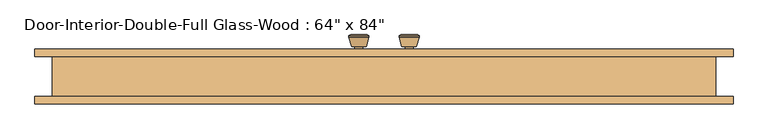
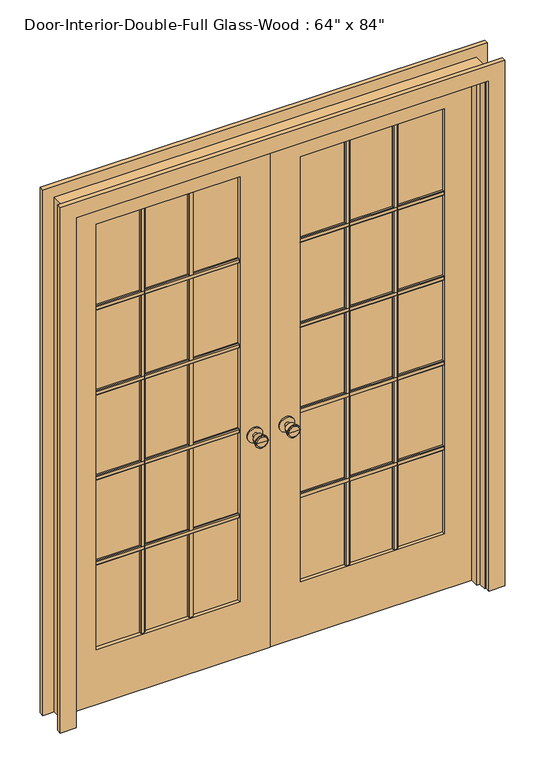
"""IFC4 building model written with IfcOpenShell, lengths in millimetres: door geometry."""

from ifc_helpers import new_model, si_unit, point, frame, frame_2d, origin, place, context, project, spatial, polyline, circle_curve, trimmed, segment, composite_curve, outline, extrude, faceted_brep, source, transform, mapped, element, save
from ifc_brep_helpers import plane_surface, cylinder_surface, revolved_surface, advanced_brep


def door_09c896ac(model_context):
    return source(origin(), model_context, "Body", "SolidModel", [
        advanced_brep(
        [(-63.5, 53.625, 914.4), (-73.5, 53.625, 914.4), (-53.5, 53.625, 914.4), (-83.9758676, 102.625, 914.4), (-63.5, 102.625, 914.4), (-43.0241324, 102.625, 914.4), (-88.5, 100.7971319, 914.4), (-38.5, 100.7971319, 914.4), (-88.5, 97.3334537, 914.4), (-38.5, 97.3334537, 914.4), (-82.136236, 72.625, 914.4), (-44.863764, 72.625, 914.4), (-73.5, 72.625, 914.4), (-53.5, 72.625, 914.4)],
        [
            (0, 1),
            (1, 2, circle_curve(frame((-63.5, 53.625, 914.4), z_axis=(0.0, -1.0, 0.0), x_axis=(1.0, 0.0, 0.0)), 10.0)),
            (2, 0),
            (2, 1, circle_curve(frame((-63.5, 53.625, 914.4), z_axis=(0.0, -1.0, 0.0), x_axis=(1.0, 0.0, 0.0)), 10.0)),
            (3, 4),
            (4, 5),
            (5, 3, circle_curve(frame((-63.5, 102.625, 914.4), z_axis=(0.0, 1.0, 0.0), x_axis=(1.0, 0.0, 0.0)), 20.4758676)),
            (3, 5, circle_curve(frame((-63.5, 102.625, 914.4), z_axis=(0.0, 1.0, 0.0), x_axis=(1.0, 0.0, 0.0)), 20.4758676)),
            (6, 3),
            (5, 7),
            (7, 6, circle_curve(frame((-63.5, 100.7971319, 914.4), z_axis=(0.0, 1.0, 0.0), x_axis=(1.0, 0.0, 0.0)), 25.0)),
            (6, 7, circle_curve(frame((-63.5, 100.7971319, 914.4), z_axis=(0.0, 1.0, 0.0), x_axis=(1.0, 0.0, 0.0)), 25.0)),
            (8, 6),
            (7, 9),
            (9, 8, circle_curve(frame((-63.5, 97.3334537, 914.4), z_axis=(0.0, 1.0, 0.0), x_axis=(1.0, 0.0, 0.0)), 25.0)),
            (8, 9, circle_curve(frame((-63.5, 97.3334537, 914.4), z_axis=(0.0, 1.0, 0.0), x_axis=(1.0, 0.0, 0.0)), 25.0)),
            (10, 8),
            (9, 11),
            (11, 10, circle_curve(frame((-63.5, 72.625, 914.4), z_axis=(0.0, 1.0, 0.0), x_axis=(1.0, 0.0, 0.0)), 18.636236)),
            (10, 11, circle_curve(frame((-63.5, 72.625, 914.4), z_axis=(0.0, 1.0, 0.0), x_axis=(1.0, 0.0, 0.0)), 18.636236)),
            (12, 10),
            (11, 13),
            (13, 12, circle_curve(frame((-63.5, 72.625, 914.4), z_axis=(0.0, 1.0, 0.0), x_axis=(1.0, 0.0, 0.0)), 10.0)),
            (12, 13, circle_curve(frame((-63.5, 72.625, 914.4), z_axis=(0.0, 1.0, 0.0), x_axis=(1.0, 0.0, 0.0)), 10.0)),
            (1, 12),
            (13, 2),
        ],
        [
            plane_surface(frame((-63.5, 53.625, 914.4), z_axis=(0.0, -1.0, 0.0), x_axis=(1.0, 0.0, 0.0))),
            plane_surface(frame((-63.5, 102.625, 914.4), z_axis=(0.0, 1.0, 0.0), x_axis=(1.0, 0.0, 0.0))),
            revolved_surface(polyline([(-43.0241324, 102.625, 914.4), (-38.5, 100.7971319, 914.4)]), (-63.5, 53.625, 914.4), (0.0, -1.0, 0.0)),
            cylinder_surface(frame((-63.5, 53.625, 914.4), z_axis=(0.0, -1.0, 0.0), x_axis=(1.0, 0.0, 0.0)), 25.0),
            revolved_surface(polyline([(-38.5, 97.3334537, 914.4), (-44.863764, 72.625, 914.4)]), (-63.5, 53.625, 914.4), (0.0, -1.0, 0.0)),
            plane_surface(frame((-63.5, 72.625, 914.4), z_axis=(0.0, -1.0, 0.0), x_axis=(1.0, 0.0, 0.0))),
            cylinder_surface(frame((-63.5, 53.625, 914.4), z_axis=(0.0, -1.0, 0.0), x_axis=(1.0, 0.0, 0.0)), 10.0),
        ],
        [
            (0, [[1, 2, 3]]),
            (0, [[-3, 4, -1]]),
            (1, [[5, 6, 7]]),
            (1, [[-6, -5, 8]]),
            (2, [[9, -7, 10, 11]]),
            (2, [[-10, -8, -9, 12]]),
            (3, [[13, -11, 14, 15]]),
            (3, [[-14, -12, -13, 16]]),
            (4, [[17, -15, 18, 19]]),
            (4, [[-18, -16, -17, 20]]),
            (5, [[21, -19, 22, 23]]),
            (5, [[-22, -20, -21, 24]]),
            (6, [[25, -23, 26, -2]]),
            (6, [[-26, -24, -25, -4]]),
        ],
    ),
        extrude(outline(composite_curve([segment(trimmed(circle_curve(frame_2d((914.4, -63.5)), 30.0), [point((914.4, -33.5))], [point((914.4, -93.5))], False, "CARTESIAN"), True, "CONTINUOUS"), segment(trimmed(circle_curve(frame_2d((914.4, -63.5)), 30.0), [point((914.4, -93.5))], [point((914.4, -33.5))], False, "CARTESIAN"), True, "CONTINUOUS")], self_intersect=False)), frame((0.0, 47.625, 0.0), z_axis=(0.0, 1.0, 0.0), x_axis=(0.0, 0.0, 1.0)), (0.0, 0.0, 1.0), 6.0),
        advanced_brep(
        [(-63.5, 6.7, 914.4), (-53.5, 6.7, 914.4), (-73.5, 6.7, 914.4), (-83.9758676, -42.3, 914.4), (-43.0241324, -42.3, 914.4), (-63.5, -42.3, 914.4), (-88.5, -40.4721319, 914.4), (-38.5, -40.4721319, 914.4), (-88.5, -37.0084537, 914.4), (-38.5, -37.0084537, 914.4), (-82.136236, -12.3, 914.4), (-44.863764, -12.3, 914.4), (-73.5, -12.3, 914.4), (-53.5, -12.3, 914.4)],
        [
            (0, 1),
            (1, 2, circle_curve(frame((-63.5, 6.7, 914.4), z_axis=(0.0, 1.0, 0.0), x_axis=(1.0, 0.0, 0.0)), 10.0)),
            (2, 0),
            (2, 1, circle_curve(frame((-63.5, 6.7, 914.4), z_axis=(0.0, 1.0, 0.0), x_axis=(1.0, 0.0, 0.0)), 10.0)),
            (3, 4, circle_curve(frame((-63.5, -42.3, 914.4), z_axis=(0.0, -1.0, 0.0), x_axis=(1.0, 0.0, 0.0)), 20.4758676)),
            (4, 5),
            (5, 3),
            (4, 3, circle_curve(frame((-63.5, -42.3, 914.4), z_axis=(0.0, -1.0, 0.0), x_axis=(1.0, 0.0, 0.0)), 20.4758676)),
            (6, 7, circle_curve(frame((-63.5, -40.4721319, 914.4), z_axis=(0.0, -1.0, 0.0), x_axis=(1.0, 0.0, 0.0)), 25.0)),
            (7, 4),
            (3, 6),
            (7, 6, circle_curve(frame((-63.5, -40.4721319, 914.4), z_axis=(0.0, -1.0, 0.0), x_axis=(1.0, 0.0, 0.0)), 25.0)),
            (8, 9, circle_curve(frame((-63.5, -37.0084537, 914.4), z_axis=(0.0, -1.0, 0.0), x_axis=(1.0, 0.0, 0.0)), 25.0)),
            (9, 7),
            (6, 8),
            (9, 8, circle_curve(frame((-63.5, -37.0084537, 914.4), z_axis=(0.0, -1.0, 0.0), x_axis=(1.0, 0.0, 0.0)), 25.0)),
            (10, 11, circle_curve(frame((-63.5, -12.3, 914.4), z_axis=(0.0, -1.0, 0.0), x_axis=(1.0, 0.0, 0.0)), 18.636236)),
            (11, 9),
            (8, 10),
            (11, 10, circle_curve(frame((-63.5, -12.3, 914.4), z_axis=(0.0, -1.0, 0.0), x_axis=(1.0, 0.0, 0.0)), 18.636236)),
            (12, 13, circle_curve(frame((-63.5, -12.3, 914.4), z_axis=(0.0, -1.0, 0.0), x_axis=(1.0, 0.0, 0.0)), 10.0)),
            (13, 11),
            (10, 12),
            (13, 12, circle_curve(frame((-63.5, -12.3, 914.4), z_axis=(0.0, -1.0, 0.0), x_axis=(1.0, 0.0, 0.0)), 10.0)),
            (1, 13),
            (12, 2),
        ],
        [
            plane_surface(frame((-63.5, 6.7, 914.4), z_axis=(0.0, 1.0, 0.0), x_axis=(1.0, 0.0, 0.0))),
            plane_surface(frame((-63.5, -42.3, 914.4), z_axis=(0.0, -1.0, 0.0), x_axis=(1.0, 0.0, 0.0))),
            revolved_surface(polyline([(-43.0241324, -42.3, 914.4), (-38.5, -40.4721319, 914.4)]), (-63.5, 6.7, 914.4), (0.0, 1.0, 0.0)),
            cylinder_surface(frame((-63.5, 6.7, 914.4), z_axis=(0.0, 1.0, 0.0), x_axis=(1.0, 0.0, 0.0)), 25.0),
            revolved_surface(polyline([(-38.5, -37.0084537, 914.4), (-44.863764, -12.3, 914.4)]), (-63.5, 6.7, 914.4), (0.0, 1.0, 0.0)),
            plane_surface(frame((-63.5, -12.3, 914.4), z_axis=(0.0, 1.0, 0.0), x_axis=(1.0, 0.0, 0.0))),
            cylinder_surface(frame((-63.5, 6.7, 914.4), z_axis=(0.0, 1.0, 0.0), x_axis=(1.0, 0.0, 0.0)), 10.0),
        ],
        [
            (0, [[1, 2, 3]]),
            (0, [[-3, 4, -1]]),
            (1, [[5, 6, 7]]),
            (1, [[8, -7, -6]]),
            (2, [[9, 10, -5, 11]]),
            (2, [[12, -11, -8, -10]]),
            (3, [[13, 14, -9, 15]]),
            (3, [[16, -15, -12, -14]]),
            (4, [[17, 18, -13, 19]]),
            (4, [[20, -19, -16, -18]]),
            (5, [[21, 22, -17, 23]]),
            (5, [[24, -23, -20, -22]]),
            (6, [[-2, 25, -21, 26]]),
            (6, [[-4, -26, -24, -25]]),
        ],
    ),
        extrude(outline(composite_curve([segment(trimmed(circle_curve(frame_2d((914.4, -63.5)), 30.0), [point((914.4, -33.5))], [point((914.4, -93.5))], False, "CARTESIAN"), True, "CONTINUOUS"), segment(trimmed(circle_curve(frame_2d((914.4, -63.5)), 30.0), [point((914.4, -93.5))], [point((914.4, -33.5))], False, "CARTESIAN"), True, "CONTINUOUS")], self_intersect=False)), frame((0.0, 6.7, 0.0), z_axis=(0.0, 1.0, 0.0), x_axis=(0.0, 0.0, 1.0)), (0.0, 0.0, 1.0), 6.0),
        extrude(outline(polyline([(26.67, 1667.51), (26.67, 1648.46), (20.32, 1648.46), (17.145, 1651.635), (17.145, 1664.335), (20.32, 1667.51), (26.67, 1667.51)])), frame((120.65, 0.0, 0.0), z_axis=(1.0, 0.0, 0.0), x_axis=(0.0, 1.0, 0.0)), (0.0, 0.0, 1.0), 571.5),
        extrude(outline(polyline([(26.67, 1310.9575), (26.67, 1291.9075), (20.32, 1291.9075), (17.145, 1295.0825), (17.145, 1307.7825), (20.32, 1310.9575), (26.67, 1310.9575)])), frame((120.65, 0.0, 0.0), z_axis=(1.0, 0.0, 0.0), x_axis=(0.0, 1.0, 0.0)), (0.0, 0.0, 1.0), 571.5),
        extrude(outline(polyline([(26.67, 954.405), (26.67, 935.355), (20.32, 935.355), (17.145, 938.53), (17.145, 951.23), (20.32, 954.405), (26.67, 954.405)])), frame((120.65, 0.0, 0.0), z_axis=(1.0, 0.0, 0.0), x_axis=(0.0, 1.0, 0.0)), (0.0, 0.0, 1.0), 571.5),
        extrude(outline(polyline([(26.67, 597.8525), (26.67, 578.8025), (20.32, 578.8025), (17.145, 581.9775), (17.145, 594.6775), (20.32, 597.8525), (26.67, 597.8525)])), frame((120.65, 0.0, 0.0), z_axis=(1.0, 0.0, 0.0), x_axis=(0.0, 1.0, 0.0)), (0.0, 0.0, 1.0), 571.5),
        extrude(outline(polyline([(492.125, 26.67), (511.175, 26.67), (511.175, 20.32), (508.0, 17.145), (495.3, 17.145), (492.125, 20.32), (492.125, 26.67)])), frame((0.0, 0.0, 231.775), z_axis=(0.0, 0.0, 1.0), x_axis=(1.0, 0.0, 0.0)), (0.0, 0.0, 1.0), 1782.7625),
        extrude(outline(polyline([(301.625, 26.67), (320.675, 26.67), (320.675, 20.32), (317.5, 17.145), (304.8, 17.145), (301.625, 20.32), (301.625, 26.67)])), frame((0.0, 0.0, 231.775), z_axis=(0.0, 0.0, 1.0), x_axis=(1.0, 0.0, 0.0)), (0.0, 0.0, 1.0), 1782.7625),
        extrude(outline(polyline([(33.655, 1667.51), (40.005, 1667.51), (43.18, 1664.335), (43.18, 1651.635), (40.005, 1648.46), (33.655, 1648.46), (33.655, 1667.51)])), frame((-692.15, 0.0, 0.0), z_axis=(1.0, 0.0, 0.0), x_axis=(0.0, 1.0, 0.0)), (0.0, 0.0, 1.0), 571.5),
        extrude(outline(polyline([(33.655, 1310.9575), (40.005, 1310.9575), (43.18, 1307.7825), (43.18, 1295.0825), (40.005, 1291.9075), (33.655, 1291.9075), (33.655, 1310.9575)])), frame((-692.15, 0.0, 0.0), z_axis=(1.0, 0.0, 0.0), x_axis=(0.0, 1.0, 0.0)), (0.0, 0.0, 1.0), 571.5),
        extrude(outline(polyline([(33.655, 954.405), (40.005, 954.405), (43.18, 951.23), (43.18, 938.53), (40.005, 935.355), (33.655, 935.355), (33.655, 954.405)])), frame((-692.15, 0.0, 0.0), z_axis=(1.0, 0.0, 0.0), x_axis=(0.0, 1.0, 0.0)), (0.0, 0.0, 1.0), 571.5),
        extrude(outline(polyline([(33.655, 597.8525), (40.005, 597.8525), (43.18, 594.6775), (43.18, 581.9775), (40.005, 578.8025), (33.655, 578.8025), (33.655, 597.8525)])), frame((-692.15, 0.0, 0.0), z_axis=(1.0, 0.0, 0.0), x_axis=(0.0, 1.0, 0.0)), (0.0, 0.0, 1.0), 571.5),
        extrude(outline(polyline([(-320.675, 33.655), (-320.675, 40.005), (-317.5, 43.18), (-304.8, 43.18), (-301.625, 40.005), (-301.625, 33.655), (-320.675, 33.655)])), frame((0.0, 0.0, 231.775), z_axis=(0.0, 0.0, 1.0), x_axis=(1.0, 0.0, 0.0)), (0.0, 0.0, 1.0), 1782.7625),
        extrude(outline(polyline([(-511.175, 33.655), (-511.175, 40.005), (-508.0, 43.18), (-495.3, 43.18), (-492.125, 40.005), (-492.125, 33.655), (-511.175, 33.655)])), frame((0.0, 0.0, 231.775), z_axis=(0.0, 0.0, 1.0), x_axis=(1.0, 0.0, 0.0)), (0.0, 0.0, 1.0), 1782.7625),
        extrude(outline(polyline([(33.655, 1667.51), (40.005, 1667.51), (43.18, 1664.335), (43.18, 1651.635), (40.005, 1648.46), (33.655, 1648.46), (33.655, 1667.51)])), frame((120.65, 0.0, 0.0), z_axis=(1.0, 0.0, 0.0), x_axis=(0.0, 1.0, 0.0)), (0.0, 0.0, 1.0), 571.5),
        extrude(outline(polyline([(33.655, 1310.9575), (40.005, 1310.9575), (43.18, 1307.7825), (43.18, 1295.0825), (40.005, 1291.9075), (33.655, 1291.9075), (33.655, 1310.9575)])), frame((120.65, 0.0, 0.0), z_axis=(1.0, 0.0, 0.0), x_axis=(0.0, 1.0, 0.0)), (0.0, 0.0, 1.0), 571.5),
        extrude(outline(polyline([(33.655, 954.405), (40.005, 954.405), (43.18, 951.23), (43.18, 938.53), (40.005, 935.355), (33.655, 935.355), (33.655, 954.405)])), frame((120.65, 0.0, 0.0), z_axis=(1.0, 0.0, 0.0), x_axis=(0.0, 1.0, 0.0)), (0.0, 0.0, 1.0), 571.5),
        extrude(outline(polyline([(33.655, 597.8525), (40.005, 597.8525), (43.18, 594.6775), (43.18, 581.9775), (40.005, 578.8025), (33.655, 578.8025), (33.655, 597.8525)])), frame((120.65, 0.0, 0.0), z_axis=(1.0, 0.0, 0.0), x_axis=(0.0, 1.0, 0.0)), (0.0, 0.0, 1.0), 571.5),
        extrude(outline(polyline([(492.125, 33.655), (492.125, 40.005), (495.3, 43.18), (508.0, 43.18), (511.175, 40.005), (511.175, 33.655), (492.125, 33.655)])), frame((0.0, 0.0, 231.775), z_axis=(0.0, 0.0, 1.0), x_axis=(1.0, 0.0, 0.0)), (0.0, 0.0, 1.0), 1782.7625),
        extrude(outline(polyline([(301.625, 33.655), (301.625, 40.005), (304.8, 43.18), (317.5, 43.18), (320.675, 40.005), (320.675, 33.655), (301.625, 33.655)])), frame((0.0, 0.0, 231.775), z_axis=(0.0, 0.0, 1.0), x_axis=(1.0, 0.0, 0.0)), (0.0, 0.0, 1.0), 1782.7625),
        extrude(outline(polyline([(26.67, 1667.51), (26.67, 1648.46), (20.32, 1648.46), (17.145, 1651.635), (17.145, 1664.335), (20.32, 1667.51), (26.67, 1667.51)])), frame((-692.15, 0.0, 0.0), z_axis=(1.0, 0.0, 0.0), x_axis=(0.0, 1.0, 0.0)), (0.0, 0.0, 1.0), 571.5),
        extrude(outline(polyline([(26.67, 1310.9575), (26.67, 1291.9075), (20.32, 1291.9075), (17.145, 1295.0825), (17.145, 1307.7825), (20.32, 1310.9575), (26.67, 1310.9575)])), frame((-692.15, 0.0, 0.0), z_axis=(1.0, 0.0, 0.0), x_axis=(0.0, 1.0, 0.0)), (0.0, 0.0, 1.0), 571.5),
        extrude(outline(polyline([(26.67, 954.405), (26.67, 935.355), (20.32, 935.355), (17.145, 938.53), (17.145, 951.23), (20.32, 954.405), (26.67, 954.405)])), frame((-692.15, 0.0, 0.0), z_axis=(1.0, 0.0, 0.0), x_axis=(0.0, 1.0, 0.0)), (0.0, 0.0, 1.0), 571.5),
        extrude(outline(polyline([(26.67, 597.8525), (26.67, 578.8025), (20.32, 578.8025), (17.145, 581.9775), (17.145, 594.6775), (20.32, 597.8525), (26.67, 597.8525)])), frame((-692.15, 0.0, 0.0), z_axis=(1.0, 0.0, 0.0), x_axis=(0.0, 1.0, 0.0)), (0.0, 0.0, 1.0), 571.5),
        extrude(outline(polyline([(-320.675, 26.67), (-301.625, 26.67), (-301.625, 20.32), (-304.8, 17.145), (-317.5, 17.145), (-320.675, 20.32), (-320.675, 26.67)])), frame((0.0, 0.0, 231.775), z_axis=(0.0, 0.0, 1.0), x_axis=(1.0, 0.0, 0.0)), (0.0, 0.0, 1.0), 1782.7625),
        extrude(outline(polyline([(-511.175, 26.67), (-492.125, 26.67), (-492.125, 20.32), (-495.3, 17.145), (-508.0, 17.145), (-511.175, 20.32), (-511.175, 26.67)])), frame((0.0, 0.0, 231.775), z_axis=(0.0, 0.0, 1.0), x_axis=(1.0, 0.0, 0.0)), (0.0, 0.0, 1.0), 1782.7625),
        advanced_brep(
        [(63.5, 6.7, 914.4), (73.5, 6.7, 914.4), (53.5, 6.7, 914.4), (83.9758676, -42.3, 914.4), (63.5, -42.3, 914.4), (43.0241324, -42.3, 914.4), (88.5, -40.4721319, 914.4), (38.5, -40.4721319, 914.4), (88.5, -37.0084537, 914.4), (38.5, -37.0084537, 914.4), (82.136236, -12.3, 914.4), (44.863764, -12.3, 914.4), (73.5, -12.3, 914.4), (53.5, -12.3, 914.4)],
        [
            (0, 1),
            (1, 2, circle_curve(frame((63.5, 6.7, 914.4), z_axis=(0.0, 1.0, 0.0), x_axis=(-1.0, 0.0, 0.0)), 10.0)),
            (2, 0),
            (2, 1, circle_curve(frame((63.5, 6.7, 914.4), z_axis=(0.0, 1.0, 0.0), x_axis=(-1.0, 0.0, 0.0)), 10.0)),
            (3, 4),
            (4, 5),
            (5, 3, circle_curve(frame((63.5, -42.3, 914.4), z_axis=(0.0, -1.0, 0.0), x_axis=(-1.0, 0.0, 0.0)), 20.4758676)),
            (3, 5, circle_curve(frame((63.5, -42.3, 914.4), z_axis=(0.0, -1.0, 0.0), x_axis=(-1.0, 0.0, 0.0)), 20.4758676)),
            (6, 3),
            (5, 7),
            (7, 6, circle_curve(frame((63.5, -40.4721319, 914.4), z_axis=(0.0, -1.0, 0.0), x_axis=(-1.0, 0.0, 0.0)), 25.0)),
            (6, 7, circle_curve(frame((63.5, -40.4721319, 914.4), z_axis=(0.0, -1.0, 0.0), x_axis=(-1.0, 0.0, 0.0)), 25.0)),
            (8, 6),
            (7, 9),
            (9, 8, circle_curve(frame((63.5, -37.0084537, 914.4), z_axis=(0.0, -1.0, 0.0), x_axis=(-1.0, 0.0, 0.0)), 25.0)),
            (8, 9, circle_curve(frame((63.5, -37.0084537, 914.4), z_axis=(0.0, -1.0, 0.0), x_axis=(-1.0, 0.0, 0.0)), 25.0)),
            (10, 8),
            (9, 11),
            (11, 10, circle_curve(frame((63.5, -12.3, 914.4), z_axis=(0.0, -1.0, 0.0), x_axis=(-1.0, 0.0, 0.0)), 18.636236)),
            (10, 11, circle_curve(frame((63.5, -12.3, 914.4), z_axis=(0.0, -1.0, 0.0), x_axis=(-1.0, 0.0, 0.0)), 18.636236)),
            (12, 10),
            (11, 13),
            (13, 12, circle_curve(frame((63.5, -12.3, 914.4), z_axis=(0.0, -1.0, 0.0), x_axis=(-1.0, 0.0, 0.0)), 10.0)),
            (12, 13, circle_curve(frame((63.5, -12.3, 914.4), z_axis=(0.0, -1.0, 0.0), x_axis=(-1.0, 0.0, 0.0)), 10.0)),
            (1, 12),
            (13, 2),
        ],
        [
            plane_surface(frame((63.5, 6.7, 914.4), z_axis=(0.0, 1.0, 0.0), x_axis=(-1.0, 0.0, 0.0))),
            plane_surface(frame((63.5, -42.3, 914.4), z_axis=(0.0, -1.0, 0.0), x_axis=(-1.0, 0.0, 0.0))),
            revolved_surface(polyline([(43.0241324, -42.3, 914.4), (38.5, -40.4721319, 914.4)]), (63.5, 6.7, 914.4), (0.0, 1.0, 0.0)),
            cylinder_surface(frame((63.5, 6.7, 914.4), z_axis=(0.0, 1.0, 0.0), x_axis=(-1.0, 0.0, 0.0)), 25.0),
            revolved_surface(polyline([(38.5, -37.0084537, 914.4), (44.863764, -12.3, 914.4)]), (63.5, 6.7, 914.4), (0.0, 1.0, 0.0)),
            plane_surface(frame((63.5, -12.3, 914.4), z_axis=(0.0, 1.0, 0.0), x_axis=(-1.0, 0.0, 0.0))),
            cylinder_surface(frame((63.5, 6.7, 914.4), z_axis=(0.0, 1.0, 0.0), x_axis=(-1.0, 0.0, 0.0)), 10.0),
        ],
        [
            (0, [[1, 2, 3]]),
            (0, [[-3, 4, -1]]),
            (1, [[5, 6, 7]]),
            (1, [[-6, -5, 8]]),
            (2, [[9, -7, 10, 11]]),
            (2, [[-10, -8, -9, 12]]),
            (3, [[13, -11, 14, 15]]),
            (3, [[-14, -12, -13, 16]]),
            (4, [[17, -15, 18, 19]]),
            (4, [[-18, -16, -17, 20]]),
            (5, [[21, -19, 22, 23]]),
            (5, [[-22, -20, -21, 24]]),
            (6, [[25, -23, 26, -2]]),
            (6, [[-26, -24, -25, -4]]),
        ],
    ),
        extrude(outline(composite_curve([segment(trimmed(circle_curve(frame_2d((914.4, 63.5)), 30.0), [point((914.4, 33.5))], [point((914.4, 93.5))], False, "CARTESIAN"), True, "CONTINUOUS"), segment(trimmed(circle_curve(frame_2d((914.4, 63.5)), 30.0), [point((914.4, 93.5))], [point((914.4, 33.5))], False, "CARTESIAN"), True, "CONTINUOUS")], self_intersect=False)), frame((0.0, 6.7, 0.0), z_axis=(0.0, 1.0, 0.0), x_axis=(0.0, 0.0, 1.0)), (0.0, 0.0, 1.0), 6.0),
        advanced_brep(
        [(63.5, 53.625, 914.4), (53.5, 53.625, 914.4), (73.5, 53.625, 914.4), (83.9758676, 102.625, 914.4), (43.0241324, 102.625, 914.4), (63.5, 102.625, 914.4), (88.5, 100.7971319, 914.4), (38.5, 100.7971319, 914.4), (88.5, 97.3334537, 914.4), (38.5, 97.3334537, 914.4), (82.136236, 72.625, 914.4), (44.863764, 72.625, 914.4), (73.5, 72.625, 914.4), (53.5, 72.625, 914.4)],
        [
            (0, 1),
            (1, 2, circle_curve(frame((63.5, 53.625, 914.4), z_axis=(0.0, -1.0, 0.0), x_axis=(-1.0, 0.0, 0.0)), 10.0)),
            (2, 0),
            (2, 1, circle_curve(frame((63.5, 53.625, 914.4), z_axis=(0.0, -1.0, 0.0), x_axis=(-1.0, 0.0, 0.0)), 10.0)),
            (3, 4, circle_curve(frame((63.5, 102.625, 914.4), z_axis=(0.0, 1.0, 0.0), x_axis=(-1.0, 0.0, 0.0)), 20.4758676)),
            (4, 5),
            (5, 3),
            (4, 3, circle_curve(frame((63.5, 102.625, 914.4), z_axis=(0.0, 1.0, 0.0), x_axis=(-1.0, 0.0, 0.0)), 20.4758676)),
            (6, 7, circle_curve(frame((63.5, 100.7971319, 914.4), z_axis=(0.0, 1.0, 0.0), x_axis=(-1.0, 0.0, 0.0)), 25.0)),
            (7, 4),
            (3, 6),
            (7, 6, circle_curve(frame((63.5, 100.7971319, 914.4), z_axis=(0.0, 1.0, 0.0), x_axis=(-1.0, 0.0, 0.0)), 25.0)),
            (8, 9, circle_curve(frame((63.5, 97.3334537, 914.4), z_axis=(0.0, 1.0, 0.0), x_axis=(-1.0, 0.0, 0.0)), 25.0)),
            (9, 7),
            (6, 8),
            (9, 8, circle_curve(frame((63.5, 97.3334537, 914.4), z_axis=(0.0, 1.0, 0.0), x_axis=(-1.0, 0.0, 0.0)), 25.0)),
            (10, 11, circle_curve(frame((63.5, 72.625, 914.4), z_axis=(0.0, 1.0, 0.0), x_axis=(-1.0, 0.0, 0.0)), 18.636236)),
            (11, 9),
            (8, 10),
            (11, 10, circle_curve(frame((63.5, 72.625, 914.4), z_axis=(0.0, 1.0, 0.0), x_axis=(-1.0, 0.0, 0.0)), 18.636236)),
            (12, 13, circle_curve(frame((63.5, 72.625, 914.4), z_axis=(0.0, 1.0, 0.0), x_axis=(-1.0, 0.0, 0.0)), 10.0)),
            (13, 11),
            (10, 12),
            (13, 12, circle_curve(frame((63.5, 72.625, 914.4), z_axis=(0.0, 1.0, 0.0), x_axis=(-1.0, 0.0, 0.0)), 10.0)),
            (1, 13),
            (12, 2),
        ],
        [
            plane_surface(frame((63.5, 53.625, 914.4), z_axis=(0.0, -1.0, 0.0), x_axis=(-1.0, 0.0, 0.0))),
            plane_surface(frame((63.5, 102.625, 914.4), z_axis=(0.0, 1.0, 0.0), x_axis=(-1.0, 0.0, 0.0))),
            revolved_surface(polyline([(43.0241324, 102.625, 914.4), (38.5, 100.7971319, 914.4)]), (63.5, 53.625, 914.4), (0.0, -1.0, 0.0)),
            cylinder_surface(frame((63.5, 53.625, 914.4), z_axis=(0.0, -1.0, 0.0), x_axis=(-1.0, 0.0, 0.0)), 25.0),
            revolved_surface(polyline([(38.5, 97.3334537, 914.4), (44.863764, 72.625, 914.4)]), (63.5, 53.625, 914.4), (0.0, -1.0, 0.0)),
            plane_surface(frame((63.5, 72.625, 914.4), z_axis=(0.0, -1.0, 0.0), x_axis=(-1.0, 0.0, 0.0))),
            cylinder_surface(frame((63.5, 53.625, 914.4), z_axis=(0.0, -1.0, 0.0), x_axis=(-1.0, 0.0, 0.0)), 10.0),
        ],
        [
            (0, [[1, 2, 3]]),
            (0, [[-3, 4, -1]]),
            (1, [[5, 6, 7]]),
            (1, [[8, -7, -6]]),
            (2, [[9, 10, -5, 11]]),
            (2, [[12, -11, -8, -10]]),
            (3, [[13, 14, -9, 15]]),
            (3, [[16, -15, -12, -14]]),
            (4, [[17, 18, -13, 19]]),
            (4, [[20, -19, -16, -18]]),
            (5, [[21, 22, -17, 23]]),
            (5, [[24, -23, -20, -22]]),
            (6, [[-2, 25, -21, 26]]),
            (6, [[-4, -26, -24, -25]]),
        ],
    ),
        extrude(outline(composite_curve([segment(trimmed(circle_curve(frame_2d((914.4, 63.5)), 30.0), [point((914.4, 33.5))], [point((914.4, 93.5))], False, "CARTESIAN"), True, "CONTINUOUS"), segment(trimmed(circle_curve(frame_2d((914.4, 63.5)), 30.0), [point((914.4, 93.5))], [point((914.4, 33.5))], False, "CARTESIAN"), True, "CONTINUOUS")], self_intersect=False)), frame((0.0, 47.625, 0.0), z_axis=(0.0, 1.0, 0.0), x_axis=(0.0, 0.0, 1.0)), (0.0, 0.0, 1.0), 6.0),
        extrude(outline(polyline([(0.0, 819.15), (0.0, 882.65), (2203.45, 882.65), (2203.45, -882.65), (0.0, -882.65), (0.0, -819.15), (2139.95, -819.15), (2139.95, 819.15), (0.0, 819.15)])), frame((0.0, -73.025, 0.0), z_axis=(0.0, 1.0, 0.0), x_axis=(0.0, 0.0, 1.0)), (0.0, 0.0, 1.0), 19.05),
        extrude(outline(polyline([(0.0, 819.15), (0.0, 882.65), (2203.45, 882.65), (2203.45, -882.65), (0.0, -882.65), (0.0, -819.15), (2139.95, -819.15), (2139.95, 819.15), (0.0, 819.15)])), frame((0.0, 47.625, 0.0), z_axis=(0.0, 1.0, 0.0), x_axis=(0.0, 0.0, 1.0)), (0.0, 0.0, 1.0), 19.05),
        faceted_brep([(838.2, 47.625, 0.0), (838.2, -53.975, 0.0), (812.8, -53.975, 0.0), (812.8, -22.225, 0.0), (800.1, -22.225, 0.0), (800.1, 12.7, 0.0), (812.8, 12.7, 0.0), (812.8, 47.625, 0.0), (838.2, 47.625, 2159.0), (838.2, -53.975, 2159.0), (-838.2, -53.975, 2159.0), (-838.2, -53.975, 0.0), (-812.8, -53.975, 0.0), (-812.8, -53.975, 2133.6), (812.8, -53.975, 2133.6), (812.8, -22.225, 2133.6), (-812.8, -22.225, 2133.6), (-812.8, -22.225, 0.0), (-800.1, -22.225, 0.0), (-800.1, -22.225, 2120.9), (800.1, -22.225, 2120.9), (800.1, 12.7, 2120.9), (1.5875, 12.7, 2120.9), (-1.6019111, 12.7, 2120.9), (-800.1, 12.7, 2120.9), (-800.1, 12.7, 0.0), (-812.8, 12.7, 0.0), (-812.8, 12.7, 2133.6), (-1.6019111, 12.7, 2133.6), (1.5875, 12.7, 2133.6), (812.8, 12.7, 2133.6), (812.8, 47.625, 2133.6), (1.5875, 47.625, 2133.6), (-1.6019111, 47.625, 2133.6), (-812.8, 47.625, 2133.6), (-812.8, 47.625, 0.0), (-838.2, 47.625, 0.0), (-838.2, 47.625, 2159.0)], [[[0, 1, 2, 3, 4, 5, 6, 7]], [[1, 0, 8, 9]], [[2, 1, 9, 10, 11, 12, 13, 14]], [[3, 2, 14, 15]], [[4, 3, 15, 16, 17, 18, 19, 20]], [[5, 4, 20, 21]], [[6, 5, 21, 22, 23, 24, 25, 26, 27, 28, 29, 30]], [[7, 6, 30, 31]], [[0, 7, 31, 32, 33, 34, 35, 36, 37, 8]], [[9, 8, 37, 10]], [[14, 13, 16, 15]], [[20, 19, 24, 23, 22, 21]], [[31, 30, 29, 28, 27, 34, 33, 32]], [[12, 11, 36, 35, 26, 25, 18, 17]], [[11, 10, 37, 36]], [[13, 12, 17, 16]], [[19, 18, 25, 24]], [[27, 26, 35, 34]]]),
        extrude(outline(polyline([(2133.6, -812.8), (0.0, -812.8), (0.0, -1.6019111), (2133.6, -1.6019111), (2133.6, -812.8)]), holes=[polyline([(231.775, -692.15), (2014.5375, -692.15), (2014.5375, -120.65), (231.775, -120.65), (231.775, -692.15)])]), frame((0.0, 12.7, 0.0), z_axis=(0.0, 1.0, 0.0), x_axis=(0.0, 0.0, 1.0)), (0.0, 0.0, 1.0), 34.925),
        extrude(outline(polyline([(0.0, 812.8), (2133.6, 812.8), (2133.6, 1.5875), (0.0, 1.5875), (0.0, 812.8)]), holes=[polyline([(2014.5375, 120.65), (2014.5375, 692.15), (231.775, 692.15), (231.775, 120.65), (2014.5375, 120.65)])]), frame((0.0, 12.7, 0.0), z_axis=(0.0, 1.0, 0.0), x_axis=(0.0, 0.0, 1.0)), (0.0, 0.0, 1.0), 34.925),
        extrude(outline(polyline([(692.15, 26.67), (120.65, 26.67), (120.65, 33.655), (692.15, 33.655), (692.15, 26.67)])), frame((0.0, 0.0, 231.775), z_axis=(0.0, 0.0, 1.0), x_axis=(1.0, 0.0, 0.0)), (0.0, 0.0, 1.0), 1782.7625),
        extrude(outline(polyline([(-120.65, 26.67), (-692.15, 26.67), (-692.15, 33.655), (-120.65, 33.655), (-120.65, 26.67)])), frame((0.0, 0.0, 231.775), z_axis=(0.0, 0.0, 1.0), x_axis=(1.0, 0.0, 0.0)), (0.0, 0.0, 1.0), 1782.7625),
    ])


if __name__ == "__main__":
    model = new_model("IFC4")
    model_context = context("Model", 3, world=origin())
    ifc_project = project(units=[si_unit("LENGTHUNIT", "METRE", prefix="MILLI")], contexts=[model_context])
    site = spatial("IfcSite", under=ifc_project)
    building = spatial("IfcBuilding", under=site)
    placement = place(None, origin())
    door_shape = door_09c896ac(model_context)
    element("IfcDoor", 1, ObjectType="Door-Interior-Double-Full Glass-Wood : 64\" x 84\"", at=placement, inside=building, context=model_context, shape_type="MappedRepresentation", body=[
        mapped(door_shape, transform((0.0, 0.0, 0.0), x_axis=(1.0, 0.0, 0.0), y_axis=(0.0, 1.0, 0.0), z_axis=(0.0, 0.0, 1.0))),
    ])
    save(model, "model.ifc")

# Revit data of these elements
# Type "Door-Interior-Double-Full Glass-Wood : 64\" x 84\""
#   Type Mark = "8"
#   Assembly Code = "C1020300"
#   Analytic Construction = "French door, wood frame with single glass"
#   Top Rail = 0' - 4 11/16"
#   Thickness = 0' - 1 3/8"
#   Thermal Resistance (R) = 1.0696 (h·ft²·°F)/BTU
#   Swing Angle [instance default] = 90.00°
#   Stiles = 0' - 4 3/4"
#   Rough Width = 5' - 6"
#   Rough Height = 7' - 1"
#   Panel Width = 2' - 8"
#   Height = 7' - 0"
#   Width = 5' - 4"
#   Heat Transfer Coefficient (U) = 0.9350 BTU/(h·ft²·°F)
#   Bottom Rail = 0' - 9 1/8"
#   Show Grill [instance default] = yes
#   Trim Material = Cherry
#   Panel Material = Cherry
#   Frame Material = Cherry
#   Door Handle Material = Aluminum
#   Visual Light Transmittance = 0
#   Solar Heat Gain Coefficient = 0
#   Wall Closure = (empty or 0)
#   Function = (empty or 0)
# Element 1 (IfcDoor, "Door-Interior-Double-Full Glass-Wood : 64\" x 84\"")
#   Materials on its faces: "Cherry", "Aluminum", "Glass"
# Materials
#   "Cherry": class "Wood", colour RGB 226 177 128, transparency 0, Description = "Prunus Serotina", Cost = 0
#   "Aluminum": class "Metal", colour RGB 247 247 247, transparency 0, Description = "Aluminum 6061", Cost = 0
#   "Glass": class "Glass", colour RGB 0 128 192, transparency 0.75, Description = "Soda Lime Glass", Cost = 0
